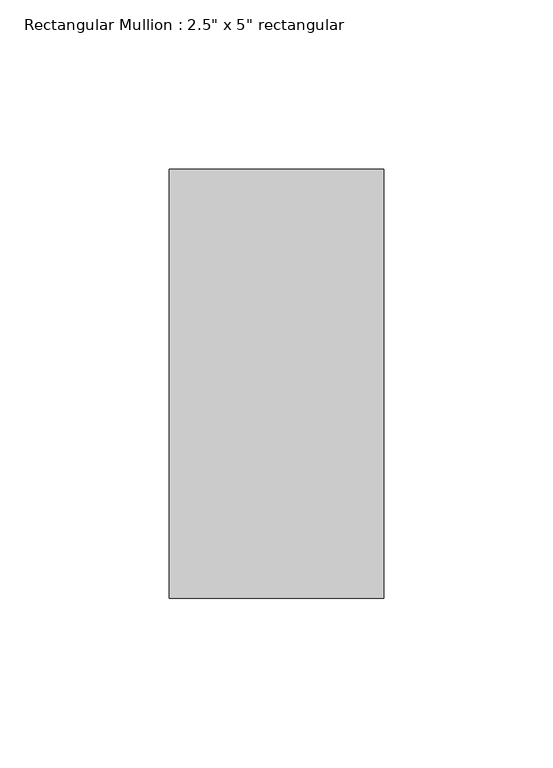
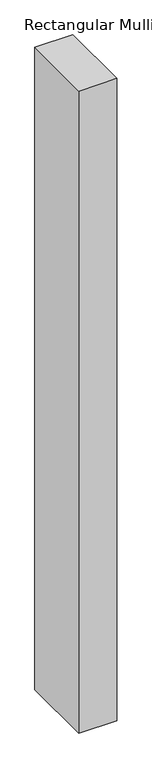
"""IFC4 building model written with IfcOpenShell, lengths in millimetres: member geometry."""

from ifc_helpers import new_model, si_unit, frame, origin, place, context, project, spatial, polyline, outline, extrude, source, transform, mapped, element, save


def member_368818a6(model_context):
    return source(origin(), model_context, "Body", "SweptSolid", [
        extrude(outline(polyline([(31.75, 63.5), (31.75, -63.5), (-31.75, -63.5), (-31.75, 63.5), (31.75, 63.5)])), frame((0.0, 0.0, -1135.8413496), z_axis=(0.0, 0.0, 1.0), x_axis=(1.0, 0.0, 0.0)), (0.0, 0.0, 1.0), 1135.8413496),
    ])


if __name__ == "__main__":
    model = new_model("IFC4")
    model_context = context("Model", 3, world=origin())
    ifc_project = project(units=[si_unit("LENGTHUNIT", "METRE", prefix="MILLI")], contexts=[model_context])
    site = spatial("IfcSite", under=ifc_project)
    building = spatial("IfcBuilding", under=site)
    placement = place(None, origin())
    member_shape = member_368818a6(model_context)
    element("IfcMember", 1, ObjectType="Rectangular Mullion : 2.5\" x 5\" rectangular", at=placement, inside=building, context=model_context, shape_type="MappedRepresentation", body=[
        mapped(member_shape, transform((0.0, 0.0, 0.0), x_axis=(1.0, 0.0, 0.0), y_axis=(0.0, 1.0, 0.0), z_axis=(0.0, 0.0, 1.0))),
    ])
    save(model, "model.ifc")

# Revit data of these elements
# Type "Rectangular Mullion : 2.5\" x 5\" rectangular"
#   built-in parameter 1007304 = 0.416667 (stored number, unit not read)
#   built-in parameter 1007301 = 0.104167 (stored number, unit not read)
#   built-in parameter 1007300 = 0.104167 (stored number, unit not read)
# Element 1 (IfcMember, "Rectangular Mullion : 2.5\" x 5\" rectangular")
#   Materials on its faces: "Aluminum"
# Materials
#   "Aluminum": class "Metal", colour RGB 247 247 247, transparency 0, Description = "Aluminum 6061", Cost = 0
